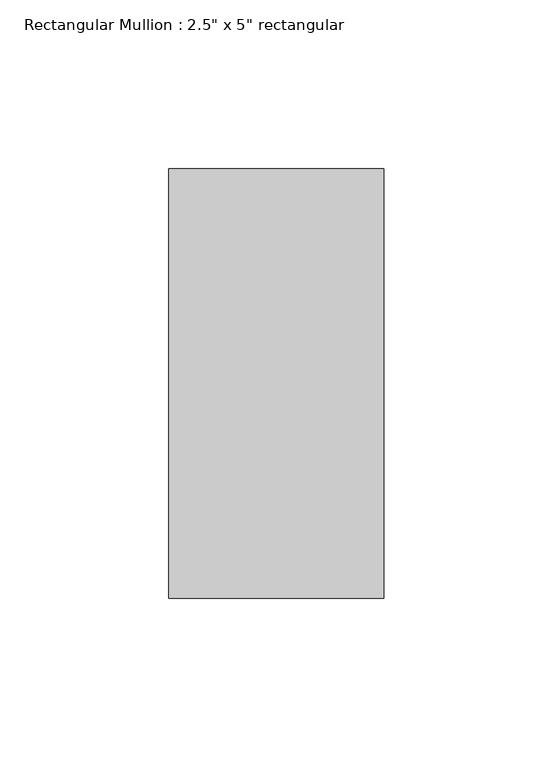
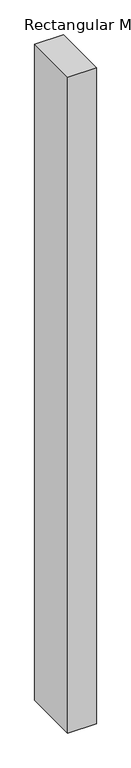
"""IFC4 building model written with IfcOpenShell, lengths in millimetres: member geometry."""

from ifc_helpers import new_model, si_unit, frame, origin, place, context, project, spatial, polyline, outline, extrude, source, transform, mapped, element, save


def member_56e9bb7d(model_context):
    return source(origin(), model_context, "Body", "SweptSolid", [
        extrude(outline(polyline([(0.0, 63.5), (0.0, -63.5), (-63.5, -63.5), (-63.5, 63.5), (0.0, 63.5)])), frame((0.0, 0.0, -1539.437083), z_axis=(0.0, 0.0, 1.0), x_axis=(1.0, 0.0, 0.0)), (0.0, 0.0, 1.0), 1539.437083),
    ])


if __name__ == "__main__":
    model = new_model("IFC4")
    model_context = context("Model", 3, world=origin())
    ifc_project = project(units=[si_unit("LENGTHUNIT", "METRE", prefix="MILLI")], contexts=[model_context])
    site = spatial("IfcSite", under=ifc_project)
    building = spatial("IfcBuilding", under=site)
    placement = place(None, origin())
    member_shape = member_56e9bb7d(model_context)
    element("IfcMember", 1, ObjectType="Rectangular Mullion : 2.5\" x 5\" rectangular", at=placement, inside=building, context=model_context, shape_type="MappedRepresentation", body=[
        mapped(member_shape, transform((0.0, 0.0, 0.0), x_axis=(1.0, 0.0, 0.0), y_axis=(0.0, 1.0, 0.0), z_axis=(0.0, 0.0, 1.0))),
    ])
    save(model, "model.ifc")

# Revit data of these elements
# Type "Rectangular Mullion : 2.5\" x 5\" rectangular"
#   built-in parameter 1007304 = 0.416667 (stored number, unit not read)
#   built-in parameter 1007301 = 0.104167 (stored number, unit not read)
#   built-in parameter 1007300 = 0.104167 (stored number, unit not read)
# Element 1 (IfcMember, "Rectangular Mullion : 2.5\" x 5\" rectangular")
#   Materials on its faces: "Aluminum"
# Materials
#   "Aluminum": class "Metal", colour RGB 247 247 247, transparency 0, Description = "Aluminum 6061", Cost = 0
